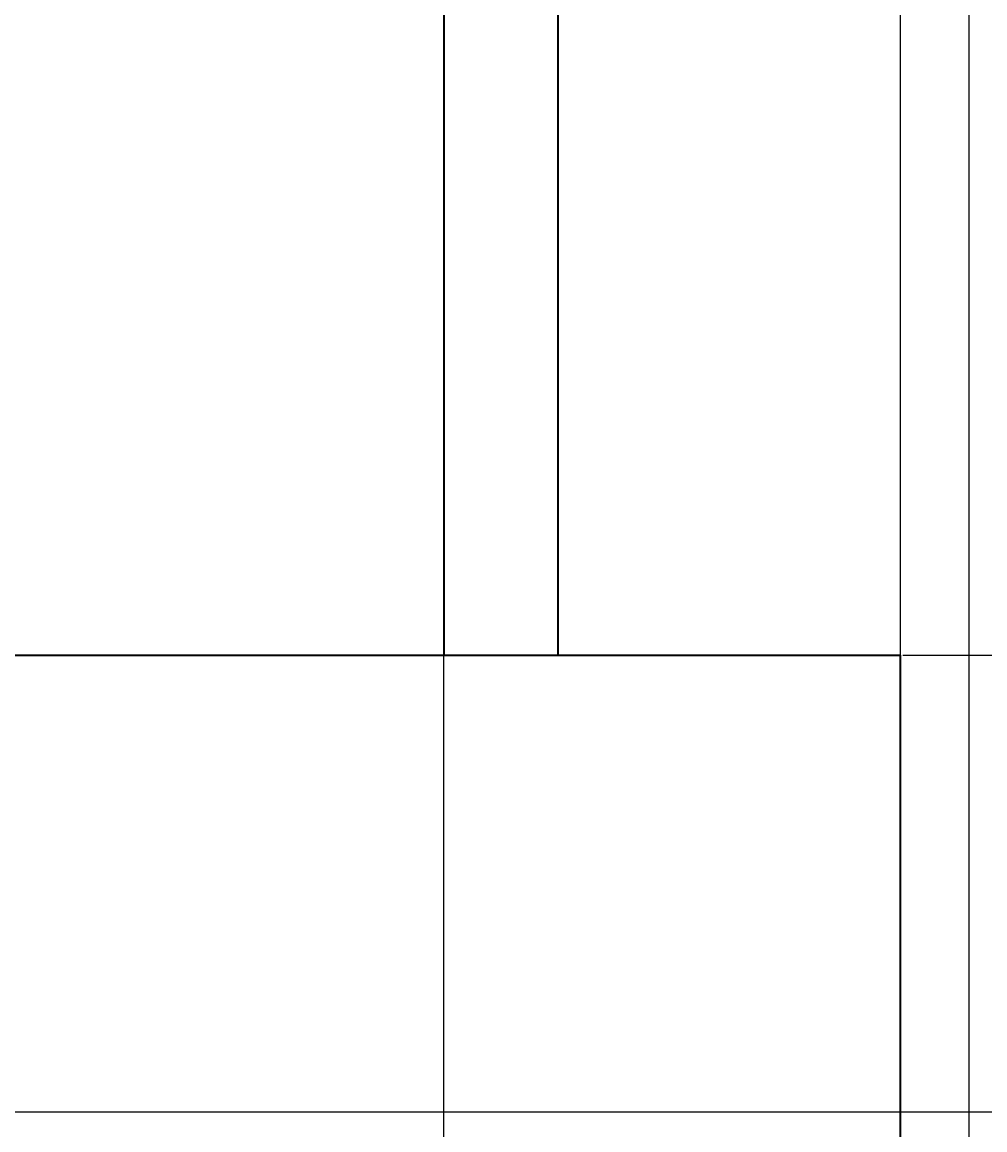
# Model space of a CAD drawing. Units: inches. Extents: x -6 to 289, y -8 to 323.
# Tile 98 of 107: x 248 to 273, y 247 to 276. Entities that reach past the tile are written whole.
import ezdxf

# ---------------------------------------------------------------- set-up
doc = ezdxf.new("R2010")
doc.units = ezdxf.units.IN
doc.header["$MEASUREMENT"] = 0
doc.layers.add('A-ANNO-DIMS', color=2, linetype='Continuous', lineweight=18)
doc.layers.add('A-ELEV', color=7, linetype='Continuous', lineweight=35)
doc.styles.get("Standard").update_dxf_attribs({"font": 'arial.ttf'})
doc.dimstyles.get("Standard").update_dxf_attribs({"dimtxt": 0.18, "dimasz": 0.18, "dimexe": 0.18, "dimexo": 0.0625, "dimgap": 0.09, "dimtad": 0, "dimtih": 1, "dimtoh": 1, "dimdec": 4, "dimzin": 0, "dimdsep": 46, "dimtxsty": 'Standard', "dimcen": 0.09, "dimadec": 0, "dimazin": 0, "dimtfac": 1, "dimtdec": 4, "dimtofl": 0, "dimtmove": 0, "dimatfit": 3, "dimfxl": 1, "dimtolj": 1, "dimtzin": 0, "dimarcsym": 0})

# ---------------------------------------------------------------- blocks, each defined once
blk = doc.blocks.new('*D15')
at = {"layer": 'A-ANNO-DIMS', "color": 0, "lineweight": -2, "transparency": 16777216}
for p, q in [((247.164, 162.411), (247.164, 322.969)), ((247.344, 322.789), (258.944, 322.789)), ((270.984, 322.789), (259.384, 322.789)), ((271.164, 7.351), (271.164, 322.969))]:
    blk.add_line(p, q, dxfattribs=at)
at = {"layer": 'A-ANNO-DIMS', "color": 0, "transparency": 16777216}
for points in [[(247.344, 322.819), (247.344, 322.759), (247.164, 322.789)], [(270.984, 322.819), (270.984, 322.759), (271.164, 322.789)]]:
    blk.add_solid(points, dxfattribs=at)
at = {"layer": 'Defpoints', "color": 0, "transparency": 16777216}
for p in [(271.164, 322.789), (247.164, 162.348), (271.164, 7.289)]:
    blk.add_point(p, dxfattribs=at)
at = {"layer": 'A-ANNO-DIMS', "color": 0, "transparency": 16777216, "insert": (259.164, 322.789), "char_height": 0.18, "attachment_point": 5}
blk.add_mtext('\\A1;24', dxfattribs=at)
blk = doc.blocks.new('*D26')
at = {"layer": 'A-ANNO-DIMS', "color": 0, "lineweight": -2, "transparency": 16777216}
for p, q in [((247.226, 247.289), (288.653, 247.289)), ((288.473, 247.109), (288.473, 237.153)), ((288.473, 226.834), (288.473, 236.789)), ((126.946, 226.654), (288.653, 226.654))]:
    blk.add_line(p, q, dxfattribs=at)
at = {"layer": 'A-ANNO-DIMS', "color": 0, "transparency": 16777216}
for points in [[(288.443, 247.109), (288.503, 247.109), (288.473, 247.289)], [(288.443, 226.834), (288.503, 226.834), (288.473, 226.654)]]:
    blk.add_solid(points, dxfattribs=at)
at = {"layer": 'Defpoints', "color": 0, "transparency": 16777216}
for p in [(247.164, 247.289), (288.473, 247.289), (126.883, 226.654)]:
    blk.add_point(p, dxfattribs=at)
at = {"layer": 'A-ANNO-DIMS', "color": 0, "transparency": 16777216, "insert": (288.473, 236.971), "char_height": 0.18, "attachment_point": 5}
blk.add_mtext('\\A1;20.635', dxfattribs=at)
blk = doc.blocks.new('*D27')
at = {"layer": 'A-ANNO-DIMS', "color": 0, "lineweight": -2, "transparency": 16777216}
for p, q in [((19.226, 307.289), (288.653, 307.289)), ((288.473, 307.109), (288.473, 277.471)), ((288.473, 247.469), (288.473, 277.107)), ((247.226, 247.289), (288.653, 247.289))]:
    blk.add_line(p, q, dxfattribs=at)
at = {"layer": 'A-ANNO-DIMS', "color": 0, "transparency": 16777216}
for points in [[(288.443, 307.109), (288.503, 307.109), (288.473, 307.289)], [(288.443, 247.469), (288.503, 247.469), (288.473, 247.289)]]:
    blk.add_solid(points, dxfattribs=at)
at = {"layer": 'Defpoints', "color": 0, "transparency": 16777216}
for p in [(19.164, 307.289), (288.473, 307.289), (247.164, 247.289)]:
    blk.add_point(p, dxfattribs=at)
at = {"layer": 'A-ANNO-DIMS', "color": 0, "transparency": 16777216, "insert": (288.473, 277.289), "char_height": 0.18, "attachment_point": 5}
blk.add_mtext('\\A1;60', dxfattribs=at)
blk = doc.blocks.new('*D82')
at = {"layer": 'A-ANNO-DIMS', "color": 0, "lineweight": -2, "transparency": 16777216}
for p, q in [((245.215, 66.286), (245.215, 322.969)), ((245.395, 322.789), (258.699, 322.789)), ((272.793, 322.789), (259.489, 322.789)), ((272.973, 66.286), (272.973, 322.969))]:
    blk.add_line(p, q, dxfattribs=at)
at = {"layer": 'A-ANNO-DIMS', "color": 0, "transparency": 16777216}
for points in [[(245.395, 322.819), (245.395, 322.759), (245.215, 322.789)], [(272.793, 322.819), (272.793, 322.759), (272.973, 322.789)]]:
    blk.add_solid(points, dxfattribs=at)
at = {"layer": 'Defpoints', "color": 0, "transparency": 16777216}
for p in [(272.973, 322.789), (245.215, 66.224), (272.973, 66.224)]:
    blk.add_point(p, dxfattribs=at)
at = {"layer": 'A-ANNO-DIMS', "color": 0, "transparency": 16777216, "insert": (259.094, 322.789), "char_height": 0.18, "attachment_point": 5}
blk.add_mtext('\\A1;27.76', dxfattribs=at)
blk = doc.blocks.new('*D100')
at = {"layer": 'A-ANNO-DIMS', "color": 0, "lineweight": -2, "transparency": 16777216}
for p, q in [((247.164, 162.411), (247.164, 322.969)), ((247.344, 322.789), (252.954, 322.789)), ((258.984, 322.789), (253.373, 322.789)), ((259.164, 139.351), (259.164, 322.969))]:
    blk.add_line(p, q, dxfattribs=at)
at = {"layer": 'A-ANNO-DIMS', "color": 0, "transparency": 16777216}
for points in [[(247.344, 322.819), (247.344, 322.759), (247.164, 322.789)], [(258.984, 322.819), (258.984, 322.759), (259.164, 322.789)]]:
    blk.add_solid(points, dxfattribs=at)
at = {"layer": 'Defpoints', "color": 0, "transparency": 16777216}
for p in [(259.164, 322.789), (247.164, 162.348), (259.164, 139.289)]:
    blk.add_point(p, dxfattribs=at)
at = {"layer": 'A-ANNO-DIMS', "color": 0, "transparency": 16777216, "insert": (253.164, 322.789), "char_height": 0.18, "attachment_point": 5}
blk.add_mtext('\\A1;12', dxfattribs=at)
blk = doc.blocks.new('*D112')
at = {"layer": 'A-ANNO-DIMS', "color": 0, "lineweight": -2, "transparency": 16777216}
for p, q in [((262.164, 280.105), (262.164, 322.969)), ((262.344, 322.789), (266.515, 322.789)), ((270.984, 322.789), (266.813, 322.789)), ((271.164, 259.351), (271.164, 322.969))]:
    blk.add_line(p, q, dxfattribs=at)
at = {"layer": 'A-ANNO-DIMS', "color": 0, "transparency": 16777216}
for points in [[(262.344, 322.819), (262.344, 322.759), (262.164, 322.789)], [(270.984, 322.819), (270.984, 322.759), (271.164, 322.789)]]:
    blk.add_solid(points, dxfattribs=at)
at = {"layer": 'Defpoints', "color": 0, "transparency": 16777216}
for p in [(271.164, 322.789), (262.164, 280.043), (271.164, 259.289)]:
    blk.add_point(p, dxfattribs=at)
at = {"layer": 'A-ANNO-DIMS', "color": 0, "transparency": 16777216, "insert": (266.664, 322.789), "char_height": 0.18, "attachment_point": 5}
blk.add_mtext('\\A1;9', dxfattribs=at)
blk = doc.blocks.new('*D113')
at = {"layer": 'A-ANNO-DIMS', "color": 0, "lineweight": -2, "transparency": 16777216}
for p, q in [((271.226, 259.289), (288.653, 259.289)), ((288.473, 259.109), (288.473, 253.469)), ((288.473, 247.469), (288.473, 253.108)), ((247.226, 247.289), (288.653, 247.289))]:
    blk.add_line(p, q, dxfattribs=at)
at = {"layer": 'A-ANNO-DIMS', "color": 0, "transparency": 16777216}
for points in [[(288.443, 259.109), (288.503, 259.109), (288.473, 259.289)], [(288.443, 247.469), (288.503, 247.469), (288.473, 247.289)]]:
    blk.add_solid(points, dxfattribs=at)
at = {"layer": 'Defpoints', "color": 0, "transparency": 16777216}
for p in [(271.164, 259.289), (288.473, 259.289), (247.164, 247.289)]:
    blk.add_point(p, dxfattribs=at)
at = {"layer": 'A-ANNO-DIMS', "color": 0, "transparency": 16777216, "insert": (288.473, 253.289), "char_height": 0.18, "attachment_point": 5}
blk.add_mtext('\\A1;12', dxfattribs=at)
blk = doc.blocks.new('*D114')
at = {"layer": 'A-ANNO-DIMS', "color": 0, "lineweight": -2, "transparency": 16777216}
for p, q in [((259.226, 277.043), (288.653, 277.043)), ((288.473, 276.863), (288.473, 268.348)), ((288.473, 259.469), (288.473, 267.984)), ((271.226, 259.289), (288.653, 259.289))]:
    blk.add_line(p, q, dxfattribs=at)
at = {"layer": 'A-ANNO-DIMS', "color": 0, "transparency": 16777216}
for points in [[(288.443, 276.863), (288.503, 276.863), (288.473, 277.043)], [(288.443, 259.469), (288.503, 259.469), (288.473, 259.289)]]:
    blk.add_solid(points, dxfattribs=at)
at = {"layer": 'Defpoints', "color": 0, "transparency": 16777216}
for p in [(259.164, 277.043), (288.473, 277.043), (271.164, 259.289)]:
    blk.add_point(p, dxfattribs=at)
at = {"layer": 'A-ANNO-DIMS', "color": 0, "transparency": 16777216, "insert": (288.473, 268.166), "char_height": 0.18, "attachment_point": 5}
blk.add_mtext('\\A1;17.754', dxfattribs=at)

msp = doc.modelspace()

# ---------------------------------------------------------------- linework, layer by layer
at = {"layer": 'A-ELEV'}
for p in [(115.1638, 259.2888), (271.1638, 68.4323)]:
    msp.add_line(p, (271.1638, 259.2888), dxfattribs=at)
for points in [[(115.1638, 307.2888), (115.1638, 277.0427), (259.1638, 277.0427), (259.1638, 259.2888)], [(118.1638, 307.2888), (118.1638, 280.0427), (262.1638, 280.0427), (262.1638, 259.2888)]]:
    msp.add_lwpolyline(points, dxfattribs=at)

# ---------------------------------------------------------------- dimensions: what is measured, and where the dimension line sits
at = {"layer": 'A-ANNO-DIMS'}
for base, p1, p2, override, picture, middle in [((272.9733, 322.7888), (245.2146, 66.2238), (272.9733, 66.2238), {"dimdec": 2, "dimlfac": 1, "dimrnd": 0, "dimzin": 0, "dimdsep": 46, "dimlunit": 2}, '*D82', (259.0939, 322.7888)), ((271.1638, 322.7888), (247.1638, 162.3484), (271.1638, 7.2888), {"dimdec": 0, "dimlfac": 1, "dimrnd": 0, "dimzin": 0, "dimdsep": 46, "dimlunit": 2}, '*D15', (259.1638, 322.7888)), ((259.1638, 322.7888), (247.1638, 162.3484), (259.1638, 139.2888), {"dimdec": 0, "dimlfac": 1, "dimrnd": 0, "dimzin": 0, "dimdsep": 46, "dimlunit": 2}, '*D100', (253.1638, 322.7888)), ((271.1638, 322.7888), (262.1638, 280.0427), (271.1638, 259.2888), {"dimdec": 0, "dimlfac": 1, "dimrnd": 0, "dimzin": 0, "dimdsep": 46, "dimlunit": 2}, '*D112', (266.6638, 322.7888))]:
    dim = msp.add_linear_dim(base=base, p1=p1, p2=p2, dimstyle='Standard', override=override, dxfattribs=at)
    dim.commit()
    dim.dimension.update_dxf_attribs({"geometry": picture, "text_midpoint": middle})
for base, p1, p2, override, picture, middle in [((288.4733, 307.2888), (247.1638, 247.2888), (19.1638, 307.2888), {"dimdec": 0, "dimlfac": 1, "dimrnd": 0, "dimzin": 0, "dimdsep": 46, "dimlunit": 2}, '*D27', (288.4733, 277.2888)), ((288.4733, 277.0427), (271.1638, 259.2888), (259.1638, 277.0427), {"dimdec": 3, "dimlfac": 1, "dimrnd": 0, "dimzin": 0, "dimdsep": 46, "dimlunit": 2}, '*D114', (288.4733, 268.1657)), ((288.4733, 259.2888), (247.1638, 247.2888), (271.1638, 259.2888), {"dimdec": 0, "dimlfac": 1, "dimrnd": 0, "dimzin": 0, "dimdsep": 46, "dimlunit": 2}, '*D113', (288.4733, 253.2888)), ((288.4733, 247.2888), (126.8835, 226.654), (247.1638, 247.2888), {"dimdec": 3, "dimlfac": 1, "dimrnd": 0, "dimzin": 0, "dimdsep": 46, "dimlunit": 2}, '*D26', (288.4733, 236.9714))]:
    dim = msp.add_linear_dim(base=base, p1=p1, p2=p2, angle=90, dimstyle='Standard', override=override, dxfattribs=at)
    dim.commit()
    dim.dimension.update_dxf_attribs({"geometry": picture, "text_midpoint": middle})

doc.saveas('drawing.dxf')
